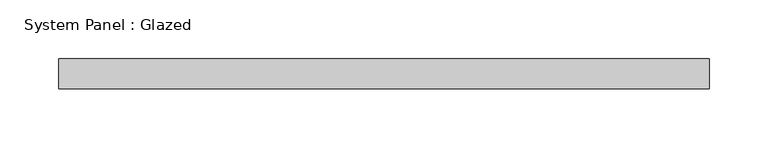
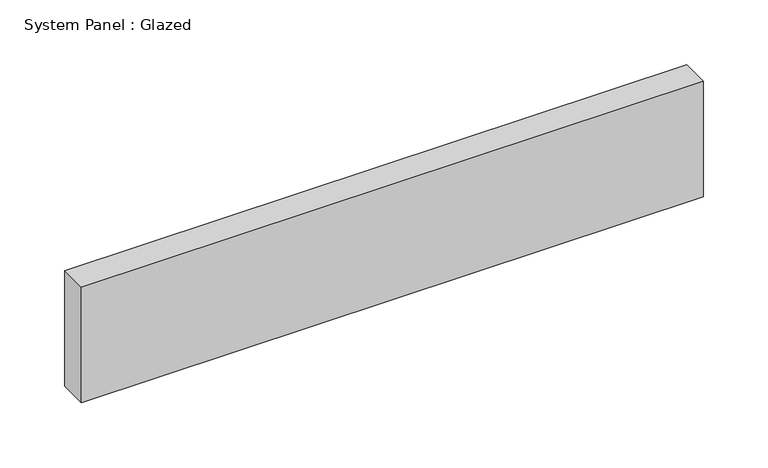
"""IFC4 building model written with IfcOpenShell, lengths in millimetres: plate geometry, System Panel : Glazed."""

from ifc_helpers import new_model, si_unit, origin, origin_with_axes, place, context, project, spatial, polyline, outline, extrude, source, transform, mapped, element, save


def system_panel_glazed_26c33eb0(model_context):
    return source(origin(), model_context, "Body", "SweptSolid", [
        extrude(outline(polyline([(276.2250002, 19.05), (-276.2250002, 19.05), (-276.2250002, 44.45), (276.2250002, 44.45), (276.2250002, 19.05)])), origin_with_axes(), (0.0, 0.0, 1.0), 108.6326151),
    ])


if __name__ == "__main__":
    model = new_model("IFC4")
    model_context = context("Model", 3, world=origin())
    ifc_project = project(units=[si_unit("LENGTHUNIT", "METRE", prefix="MILLI")], contexts=[model_context])
    site = spatial("IfcSite", under=ifc_project)
    building = spatial("IfcBuilding", under=site)
    placement = place(None, origin())
    system_panel_glazed_shape = system_panel_glazed_26c33eb0(model_context)
    element("IfcPlate", 1, ObjectType="System Panel : Glazed", at=placement, inside=building, context=model_context, shape_type="MappedRepresentation", body=[
        mapped(system_panel_glazed_shape, transform((0.0, 0.0, 0.0), x_axis=(1.0, 0.0, 0.0), y_axis=(0.0, 1.0, 0.0), z_axis=(0.0, 0.0, 1.0))),
    ])
    save(model, "model.ifc")

# Revit data of these elements
# Type "System Panel : Glazed"
#   Construction Type Id = "GSP4R"
#   Analytic Construction = "1/8 in Pilkington single glazing"
#   Visual Light Transmittance = 0.9
#   Solar Heat Gain Coefficient = 0.86
#   Heat Transfer Coefficient (U) = 1.18115 BTU/(h·ft²·°F)
#   Define Thermal Properties by = 1
# Element 1 (IfcPlate, "System Panel : Glazed")
#   Materials on its faces: "Glass"
# Materials
#   "Glass": class "Glass", colour RGB 0 128 192, transparency 0.75, Description = "Soda Lime Glass", Cost = 0
